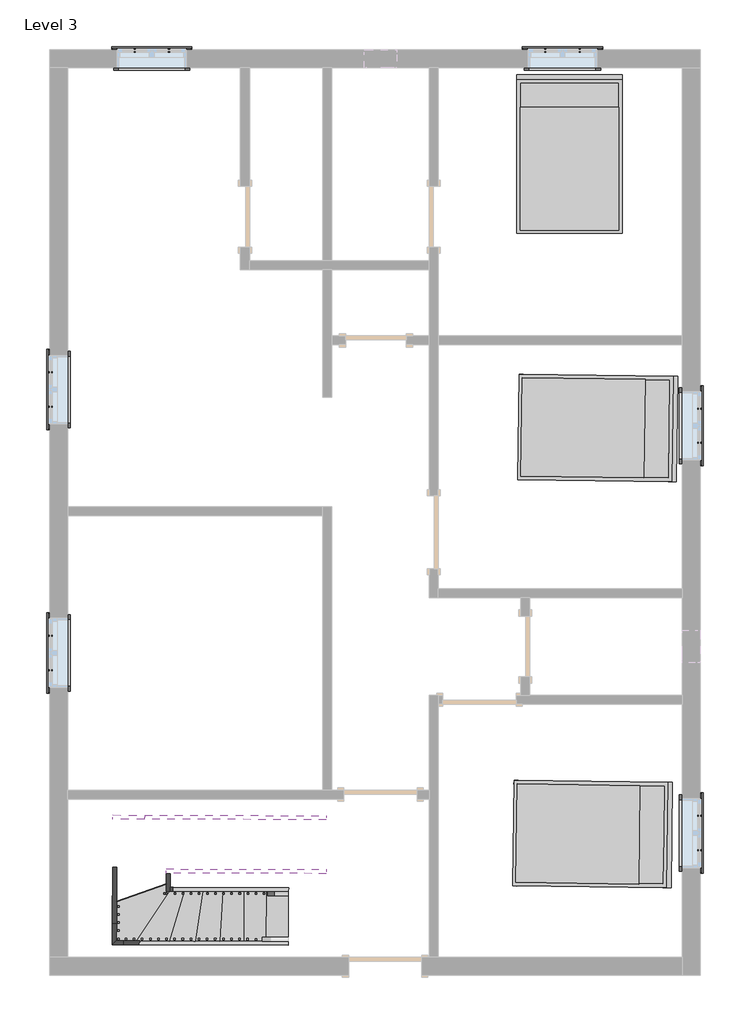
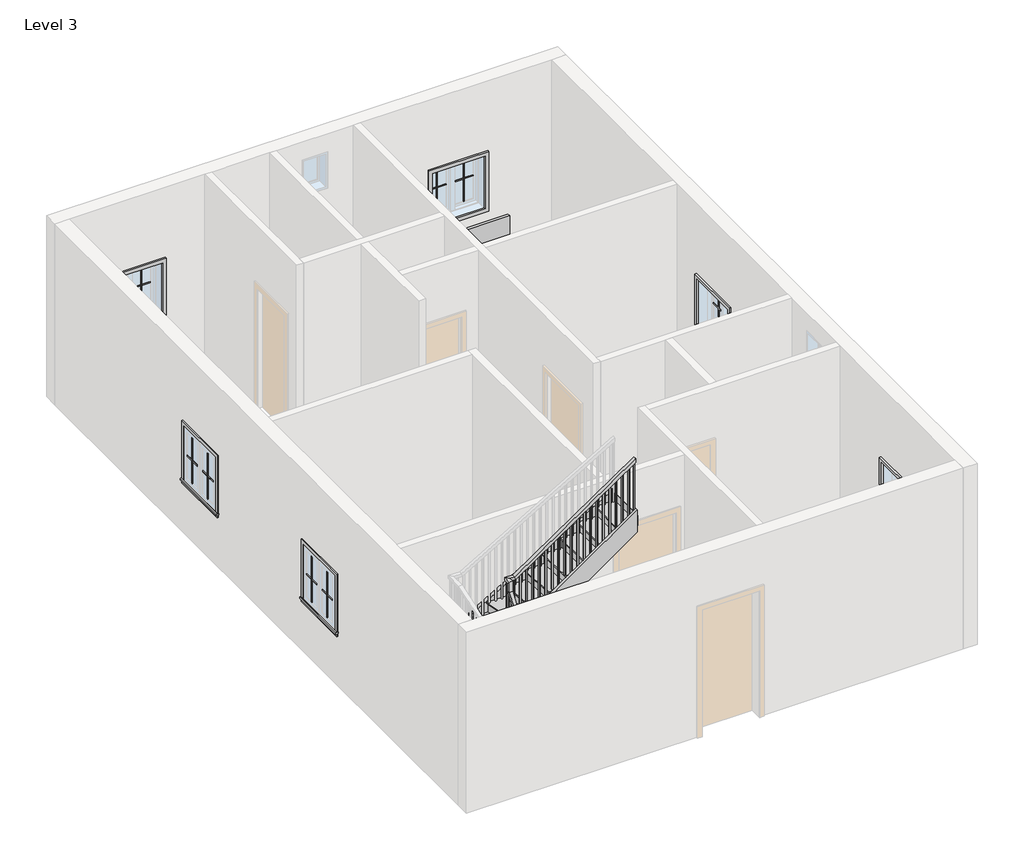
# One storey, part 3 of 3: 24 proxies, 9 members, 3 furniture elements, 1 railing, 1 stair flight.
"""IFC4 building model written with IfcOpenShell, lengths in millimetres."""

from ifc_helpers import new_model, si_unit, frame, origin, place, context, project, spatial, polyline, outline, extrude, faceted_brep, transform, mapped, element, save
from components import muntin_pattern_2x2_muntin_pattern_2x2_b3fe6957, muntin_pattern_2x2_muntin_pattern_2x2_3e0ecaf2, trim_window_exterior_flat_with_sill_41619996, trim_window_interior_flat_picture_frame_51c85655, bed_17739_bed_17739_15c61121, stair_flight_9e3aa5cb

model = new_model("IFC4")

# Units and contexts
model_context = context("Model", 3, world=origin())
ifc_project = project(units=[si_unit("LENGTHUNIT", "METRE", prefix="MILLI")], contexts=[model_context])

# Site, building, storey
site = spatial("IfcSite", under=ifc_project)
building = spatial("IfcBuilding", under=site)
storey = spatial("IfcBuildingStorey", under=building, Name="Level 3", Elevation=3200.4)

# Proxies
placement = place(None, origin())
muntin_pattern_2x2_muntin_pattern_2x2_shape = muntin_pattern_2x2_muntin_pattern_2x2_b3fe6957(model_context)
element("IfcBuildingElementProxy", 1, Name="Muntin Pattern_2x2 : Muntin Pattern_2x2", ObjectType="Muntin Pattern_2x2 : Muntin Pattern_2x2", at=placement, inside=storey, context=model_context, shape_type="MappedRepresentation", body=[
    mapped(muntin_pattern_2x2_muntin_pattern_2x2_shape, transform((873.7257686, 6321.6571212, 4184.65), x_axis=(1.0, 0.0, 0.0), y_axis=(0.0, 1.0, 0.0), z_axis=(0.0, 0.0, 1.0))),
])
element("IfcBuildingElementProxy", 2, Name="Muntin Pattern_2x2 : Muntin Pattern_2x2", ObjectType="Muntin Pattern_2x2 : Muntin Pattern_2x2", at=placement, inside=storey, context=model_context, shape_type="MappedRepresentation", body=[
    mapped(muntin_pattern_2x2_muntin_pattern_2x2_shape, transform((2802.5382686, 1840.1446212, 4184.65), x_axis=(0.0, -1.0, 0.0), y_axis=(1.0, 0.0, 0.0), z_axis=(0.0, 0.0, 1.0))),
])
element("IfcBuildingElementProxy", 3, Name="Muntin Pattern_2x2 : Muntin Pattern_2x2", ObjectType="Muntin Pattern_2x2 : Muntin Pattern_2x2", at=placement, inside=storey, context=model_context, shape_type="MappedRepresentation", body=[
    mapped(muntin_pattern_2x2_muntin_pattern_2x2_shape, transform((2802.5382686, -3255.7303788, 4184.65), x_axis=(0.0, -1.0, 0.0), y_axis=(1.0, 0.0, 0.0), z_axis=(0.0, 0.0, 1.0))),
])
element("IfcBuildingElementProxy", 4, Name="Muntin Pattern_2x2 : Muntin Pattern_2x2", ObjectType="Muntin Pattern_2x2 : Muntin Pattern_2x2", at=placement, inside=storey, context=model_context, shape_type="MappedRepresentation", body=[
    mapped(muntin_pattern_2x2_muntin_pattern_2x2_shape, transform((-4263.4242314, 6321.6571212, 4184.65), x_axis=(1.0, 0.0, 0.0), y_axis=(0.0, 1.0, 0.0), z_axis=(0.0, 0.0, 1.0))),
])
element("IfcBuildingElementProxy", 5, Name="Muntin Pattern_2x2 : Muntin Pattern_2x2", ObjectType="Muntin Pattern_2x2 : Muntin Pattern_2x2", at=placement, inside=storey, context=model_context, shape_type="MappedRepresentation", body=[
    mapped(muntin_pattern_2x2_muntin_pattern_2x2_shape, transform((-5319.1117314, 1863.8332318, 4184.65), x_axis=(0.0, 1.0, 0.0), y_axis=(-1.0, 0.0, 0.0), z_axis=(0.0, 0.0, 1.0))),
])
element("IfcBuildingElementProxy", 6, Name="Muntin Pattern_2x2 : Muntin Pattern_2x2", ObjectType="Muntin Pattern_2x2 : Muntin Pattern_2x2", at=placement, inside=storey, context=model_context, shape_type="MappedRepresentation", body=[
    mapped(muntin_pattern_2x2_muntin_pattern_2x2_shape, transform((-5319.1117314, -1431.8167682, 4184.65), x_axis=(0.0, 1.0, 0.0), y_axis=(-1.0, 0.0, 0.0), z_axis=(0.0, 0.0, 1.0))),
])
muntin_pattern_2x2_muntin_pattern_2x2_2_shape = muntin_pattern_2x2_muntin_pattern_2x2_3e0ecaf2(model_context)
element("IfcBuildingElementProxy", 7, Name="Muntin Pattern_2x2 : Muntin Pattern_2x2", ObjectType="Muntin Pattern_2x2 : Muntin Pattern_2x2", at=placement, inside=storey, context=model_context, shape_type="MappedRepresentation", body=[
    mapped(muntin_pattern_2x2_muntin_pattern_2x2_2_shape, transform((1302.3507686, 6321.6571212, 4184.65), x_axis=(-1.0, 0.0, 0.0), y_axis=(0.0, -1.0, 0.0), z_axis=(0.0, 0.0, 1.0))),
])
element("IfcBuildingElementProxy", 8, Name="Muntin Pattern_2x2 : Muntin Pattern_2x2", ObjectType="Muntin Pattern_2x2 : Muntin Pattern_2x2", at=placement, inside=storey, context=model_context, shape_type="MappedRepresentation", body=[
    mapped(muntin_pattern_2x2_muntin_pattern_2x2_2_shape, transform((2802.5382686, 1411.5196212, 4184.65), x_axis=(0.0, 1.0, 0.0), y_axis=(-1.0, 0.0, 0.0), z_axis=(0.0, 0.0, 1.0))),
])
element("IfcBuildingElementProxy", 9, Name="Muntin Pattern_2x2 : Muntin Pattern_2x2", ObjectType="Muntin Pattern_2x2 : Muntin Pattern_2x2", at=placement, inside=storey, context=model_context, shape_type="MappedRepresentation", body=[
    mapped(muntin_pattern_2x2_muntin_pattern_2x2_2_shape, transform((2802.5382686, -3684.3553788, 4184.65), x_axis=(0.0, 1.0, 0.0), y_axis=(-1.0, 0.0, 0.0), z_axis=(0.0, 0.0, 1.0))),
])
element("IfcBuildingElementProxy", 10, Name="Muntin Pattern_2x2 : Muntin Pattern_2x2", ObjectType="Muntin Pattern_2x2 : Muntin Pattern_2x2", at=placement, inside=storey, context=model_context, shape_type="MappedRepresentation", body=[
    mapped(muntin_pattern_2x2_muntin_pattern_2x2_2_shape, transform((-3834.7992314, 6321.6571212, 4184.65), x_axis=(-1.0, 0.0, 0.0), y_axis=(0.0, -1.0, 0.0), z_axis=(0.0, 0.0, 1.0))),
])
element("IfcBuildingElementProxy", 11, Name="Muntin Pattern_2x2 : Muntin Pattern_2x2", ObjectType="Muntin Pattern_2x2 : Muntin Pattern_2x2", at=placement, inside=storey, context=model_context, shape_type="MappedRepresentation", body=[
    mapped(muntin_pattern_2x2_muntin_pattern_2x2_2_shape, transform((-5319.1117314, 2292.4582318, 4184.65), x_axis=(0.0, -1.0, 0.0), y_axis=(1.0, 0.0, 0.0), z_axis=(0.0, 0.0, 1.0))),
])
element("IfcBuildingElementProxy", 12, Name="Muntin Pattern_2x2 : Muntin Pattern_2x2", ObjectType="Muntin Pattern_2x2 : Muntin Pattern_2x2", at=placement, inside=storey, context=model_context, shape_type="MappedRepresentation", body=[
    mapped(muntin_pattern_2x2_muntin_pattern_2x2_2_shape, transform((-5319.1117314, -1003.1917682, 4184.65), x_axis=(0.0, -1.0, 0.0), y_axis=(1.0, 0.0, 0.0), z_axis=(0.0, 0.0, 1.0))),
])
trim_window_exterior_flat_with_sill_shape = trim_window_exterior_flat_with_sill_41619996(model_context)
element("IfcBuildingElementProxy", 13, Name="Trim-Window-Exterior-Flat : with Sill", ObjectType="Trim-Window-Exterior-Flat : with Sill", at=placement, inside=storey, context=model_context, shape_type="MappedRepresentation", body=[
    mapped(trim_window_exterior_flat_with_sill_shape, transform((1088.0382686, 6331.1821212, 5029.2), x_axis=(-1.0, 0.0, 0.0), y_axis=(0.0, 0.0, 1.0), z_axis=(0.0, 1.0, 0.0))),
])
element("IfcBuildingElementProxy", 14, Name="Trim-Window-Exterior-Flat : with Sill", ObjectType="Trim-Window-Exterior-Flat : with Sill", at=placement, inside=storey, context=model_context, shape_type="MappedRepresentation", body=[
    mapped(trim_window_exterior_flat_with_sill_shape, transform((2812.0632686, 1625.8321212, 5029.2), x_axis=(0.0, 1.0, 0.0), y_axis=(0.0, 0.0, 1.0), z_axis=(1.0, 0.0, 0.0))),
])
element("IfcBuildingElementProxy", 15, Name="Trim-Window-Exterior-Flat : with Sill", ObjectType="Trim-Window-Exterior-Flat : with Sill", at=placement, inside=storey, context=model_context, shape_type="MappedRepresentation", body=[
    mapped(trim_window_exterior_flat_with_sill_shape, transform((2812.0632686, -3470.0428788, 5029.2), x_axis=(0.0, 1.0, 0.0), y_axis=(0.0, 0.0, 1.0), z_axis=(1.0, 0.0, 0.0))),
])
element("IfcBuildingElementProxy", 16, Name="Trim-Window-Exterior-Flat : with Sill", ObjectType="Trim-Window-Exterior-Flat : with Sill", at=placement, inside=storey, context=model_context, shape_type="MappedRepresentation", body=[
    mapped(trim_window_exterior_flat_with_sill_shape, transform((-4049.1117314, 6331.1821212, 5029.2), x_axis=(-1.0, 0.0, 0.0), y_axis=(0.0, 0.0, 1.0), z_axis=(0.0, 1.0, 0.0))),
])
element("IfcBuildingElementProxy", 17, Name="Trim-Window-Exterior-Flat : with Sill", ObjectType="Trim-Window-Exterior-Flat : with Sill", at=placement, inside=storey, context=model_context, shape_type="MappedRepresentation", body=[
    mapped(trim_window_exterior_flat_with_sill_shape, transform((-5328.6367314, 2078.1457318, 5029.2), x_axis=(0.0, -1.0, 0.0), y_axis=(0.0, 0.0, 1.0), z_axis=(-1.0, 0.0, 0.0))),
])
element("IfcBuildingElementProxy", 18, Name="Trim-Window-Exterior-Flat : with Sill", ObjectType="Trim-Window-Exterior-Flat : with Sill", at=placement, inside=storey, context=model_context, shape_type="MappedRepresentation", body=[
    mapped(trim_window_exterior_flat_with_sill_shape, transform((-5328.6367314, -1217.5042682, 5029.2), x_axis=(0.0, -1.0, 0.0), y_axis=(0.0, 0.0, 1.0), z_axis=(-1.0, 0.0, 0.0))),
])
trim_window_interior_flat_picture_frame_shape = trim_window_interior_flat_picture_frame_51c85655(model_context)
element("IfcBuildingElementProxy", 19, Name="Trim-Window-Interior-Flat : Picture Frame", ObjectType="Trim-Window-Interior-Flat : Picture Frame", at=placement, inside=storey, context=model_context, shape_type="MappedRepresentation", body=[
    mapped(trim_window_interior_flat_picture_frame_shape, transform((1088.0382686, 6102.5821212, 5029.2), x_axis=(1.0, 0.0, 0.0), y_axis=(0.0, 0.0, 1.0), z_axis=(0.0, -1.0, 0.0))),
])
element("IfcBuildingElementProxy", 20, Name="Trim-Window-Interior-Flat : Picture Frame", ObjectType="Trim-Window-Interior-Flat : Picture Frame", at=placement, inside=storey, context=model_context, shape_type="MappedRepresentation", body=[
    mapped(trim_window_interior_flat_picture_frame_shape, transform((2583.4632686, 1625.8321212, 5029.2), x_axis=(0.0, -1.0, 0.0), y_axis=(0.0, 0.0, 1.0), z_axis=(-1.0, 0.0, 0.0))),
])
element("IfcBuildingElementProxy", 21, Name="Trim-Window-Interior-Flat : Picture Frame", ObjectType="Trim-Window-Interior-Flat : Picture Frame", at=placement, inside=storey, context=model_context, shape_type="MappedRepresentation", body=[
    mapped(trim_window_interior_flat_picture_frame_shape, transform((2583.4632686, -3470.0428788, 5029.2), x_axis=(0.0, -1.0, 0.0), y_axis=(0.0, 0.0, 1.0), z_axis=(-1.0, 0.0, 0.0))),
])
element("IfcBuildingElementProxy", 22, Name="Trim-Window-Interior-Flat : Picture Frame", ObjectType="Trim-Window-Interior-Flat : Picture Frame", at=placement, inside=storey, context=model_context, shape_type="MappedRepresentation", body=[
    mapped(trim_window_interior_flat_picture_frame_shape, transform((-4049.1117314, 6102.5821212, 5029.2), x_axis=(1.0, 0.0, 0.0), y_axis=(0.0, 0.0, 1.0), z_axis=(0.0, -1.0, 0.0))),
])
element("IfcBuildingElementProxy", 23, Name="Trim-Window-Interior-Flat : Picture Frame", ObjectType="Trim-Window-Interior-Flat : Picture Frame", at=placement, inside=storey, context=model_context, shape_type="MappedRepresentation", body=[
    mapped(trim_window_interior_flat_picture_frame_shape, transform((-5100.0367314, 2078.1457318, 5029.2), x_axis=(0.0, 1.0, 0.0), y_axis=(0.0, 0.0, 1.0), z_axis=(1.0, 0.0, 0.0))),
])
element("IfcBuildingElementProxy", 24, Name="Trim-Window-Interior-Flat : Picture Frame", ObjectType="Trim-Window-Interior-Flat : Picture Frame", at=placement, inside=storey, context=model_context, shape_type="MappedRepresentation", body=[
    mapped(trim_window_interior_flat_picture_frame_shape, transform((-5100.0367314, -1217.5042682, 5029.2), x_axis=(0.0, 1.0, 0.0), y_axis=(0.0, 0.0, 1.0), z_axis=(1.0, 0.0, 0.0))),
])

# Furniture
bed_17739_bed_17739_shape = bed_17739_bed_17739_15c61121(model_context)
element("IfcFurniture", 25, ObjectType="Bed_17739 : Bed_17739", at=placement, inside=storey, context=model_context, shape_type="MappedRepresentation", body=[
    mapped(bed_17739_bed_17739_shape, transform((1173.7632686, 4997.6821212, 3200.4), x_axis=(1.0, 0.0, 0.0), y_axis=(0.0, 1.0, 0.0), z_axis=(0.0, 0.0, 1.0))),
])
element("IfcFurniture", 26, ObjectType="Bed_17739 : Bed_17739", at=placement, inside=storey, context=model_context, shape_type="MappedRepresentation", body=[
    mapped(bed_17739_bed_17739_shape, transform((1503.3372561, 1596.4447738, 3200.4), x_axis=(-0.012740965827000846, -0.9999188306006619, 0.0), y_axis=(0.9999188306006619, -0.012740965827000846, 0.0), z_axis=(0.0, 0.0, 1.0))),
])
element("IfcFurniture", 27, ObjectType="Bed_17739 : Bed_17739", at=placement, inside=storey, context=model_context, shape_type="MappedRepresentation", body=[
    mapped(bed_17739_bed_17739_shape, transform((1438.6034215, -3483.9063624, 3200.4), x_axis=(-0.012740965827007402, -0.9999188306006618, 0.0), y_axis=(0.9999188306006618, -0.012740965827007402, 0.0), z_axis=(0.0, 0.0, 1.0))),
])

# Members
element("IfcMember", 28, ObjectType="Stringer - 2\" Width", at=placement, inside=storey, context=model_context, shape_type="SweptSolid", body=[
    extrude(outline(polyline([(-105.6436802, -202.41926), (0.0, 0.0), (2328.0658822, 0.0), (2168.9891534, -304.7999999), (90.5236019, -304.7999999), (-105.6436802, -202.41926)])), frame((-2342.1993001, -4876.8012848, 3428.7290257), z_axis=(0.0033835818014385714, 0.9999942756707126, 0.0), x_axis=(-0.8865193579369283, 0.0029996279369964417, 0.46268178074713084)), (0.0, 0.0, 1.0), 50.8),
])
element("IfcMember", 29, ObjectType="Stringer - 2\" Width", at=placement, inside=storey, context=model_context, shape_type="SweptSolid", body=[
    extrude(outline(polyline([(-4405.9028852, -4819.0182441), (-4406.0747712, -4869.8179533), (-4542.6986856, -4869.3556725), (-4491.7270905, -4818.7278493), (-4405.9028852, -4819.0182441)])), frame((0.0, 0.0, 4162.0681426), z_axis=(0.0, 0.0, 1.0), x_axis=(1.0, 0.0, 0.0)), (0.0, 0.0, 1.0), 343.8145513),
])
element("IfcMember", 30, ObjectType="Stringer - 2\" Width", at=placement, inside=storey, context=model_context, shape_type="SweptSolid", body=[
    extrude(outline(polyline([(-4491.7270905, -4818.7278493), (-4542.6986856, -4869.3556725), (-4541.8102896, -4606.7963526), (-4491.0105804, -4606.9682386), (-4491.7270905, -4818.7278493)])), frame((0.0, 0.0, 4162.0681426), z_axis=(0.0, 0.0, 1.0), x_axis=(1.0, 0.0, 0.0)), (0.0, 0.0, 1.0), 343.8145513),
])
element("IfcMember", 31, ObjectType="Stringer - 2\" Width", at=placement, inside=storey, context=model_context, shape_type="SweptSolid", body=[
    extrude(outline(polyline([(109.7110974, -325.8403301), (0.0, 0.0), (1383.9510961, 0.0), (1489.930143, -314.7561954), (1457.0104275, -325.8403301), (109.7110974, -325.8403301)])), frame((-4491.0105804, -4606.9682386, 4162.0681426), z_axis=(-0.9999942756707125, 0.003383581801438886, 0.0), x_axis=(0.0032066921171017464, 0.9477157489074122, 0.3190996339680272)), (0.0, 0.0, 1.0), 50.8),
])
element("IfcMember", 32, ObjectType="Stringer - 2\" Width", at=placement, inside=storey, context=model_context, shape_type="SweptSolid", body=[
    extrude(outline(polyline([(-4537.3723845, -3295.2041032), (-4537.2004986, -3244.404394), (-4139.0142012, -3245.7516976), (-4139.1860871, -3296.5514068), (-4537.3723845, -3295.2041032)])), frame((0.0, 0.0, 4614.1918365), z_axis=(0.0, 0.0, 1.0), x_axis=(1.0, 0.0, 0.0)), (0.0, 0.0, 1.0), 321.6135804),
])
element("IfcMember", 33, ObjectType="Stringer - 2\" Width", at=placement, inside=storey, context=model_context, shape_type="SweptSolid", body=[
    extrude(outline(polyline([(-111.9549294, -160.635527), (0.0, 0.0), (1800.2454177, 0.0), (1587.8150598, -304.8000001), (94.8955973, -304.8), (-111.9549294, -160.635527)])), frame((-2339.9228929, -4204.0248458, 3396.2000989), z_axis=(0.003383581801438833, 0.9999942756707125, 0.0), x_axis=(-0.8204010535979692, 0.0027759099650580456, 0.5717817814334486)), (0.0, 0.0, 1.0), 50.8),
])
element("IfcMember", 34, ObjectType="Stringer - 2\" Width", at=placement, inside=storey, context=model_context, shape_type="SweptSolid", body=[
    extrude(outline(polyline([(438.5777673, -304.8), (2.5808594, -1.7936294), (3.8273846, 0.0), (400.5684618, 0.0), (819.8223258, -291.370396), (810.4891046, -304.8000001), (438.5777673, -304.8)])), frame((-3816.8461303, -4199.0275266, 4086.2862902), z_axis=(-0.9999942756707125, 0.003383581801437359, 0.0), x_axis=(0.0019309727886812926, 0.5706856959500506, 0.8211663094538743)), (0.0, 0.0, 1.0), 50.8),
])
element("IfcMember", 35, ObjectType="Stringer - 2\" Width", at=placement, inside=storey, context=model_context, shape_type="SweptSolid", body=[
    extrude(outline(polyline([(213.8292849, -304.8), (0.0, 0.0), (2440.5867528, 0.0), (2654.4160377, -304.8), (213.8292849, -304.8)])), frame((-3866.8723527, -3970.2569493, 4553.4535021), z_axis=(0.003383581801438697, 0.9999942756707126, 0.0), x_axis=(0.8186346554264393, -0.0027699331781375542, 0.5743079560697587)), (0.0, 0.0, 1.0), 50.8),
])
element("IfcMember", 36, ObjectType="Stringer - 2\" Width", at=placement, inside=storey, context=model_context, shape_type="SweptSolid", body=[
    extrude(outline(polyline([(162.5062199, -277.5374274), (0.0, 0.0), (2633.4595913, 1e-07), (2795.9658112, -277.5374274), (162.5062199, -277.5374274)])), frame((-4139.1860871, -3296.5514068, 4614.1918365), z_axis=(0.0033835818014385927, 0.9999942756707125, 0.0), x_axis=(0.8629481327443969, -0.002919872311849946, 0.5052840731100094)), (0.0, 0.0, 1.0), 50.8),
])

# Railing
element("IfcRailing", 37, ObjectType="Handrail - Rectangular", at=placement, inside=storey, context=model_context, shape_type="SolidModel", body=[
    faceted_brep([(-2340.0947789, -4254.824555, 4284.1333333), (-2340.0947789, -4254.824555, 4222.7023206), (-2339.9228929, -4204.0248458, 4222.7023206), (-2339.9228929, -4204.0248458, 4284.1333333), (-3791.6181617, -4249.9131788, 5271.1092848), (-3842.4178709, -4249.7412929, 5244.2199762), (-3842.2459849, -4198.9415837, 5244.2199762), (-3791.4462757, -4199.1134696, 5271.1092848), (-1868.5796854, -3875.4177931, 7162.8), (-1868.7515713, -3926.2175023, 7162.8), (-1868.7515713, -3926.2175023, 7101.138507), (-1868.5796854, -3875.4177931, 7101.138507), (-3774.5418549, -3868.9687773, 5789.845528), (-3790.329017, -3868.9153598, 5840.645528), (-3774.7137409, -3919.7684865, 5789.845528), (-3790.500903, -3919.715069, 5840.645528), (-3791.6181617, -4249.9131788, 5487.4182666), (-3842.4178709, -4249.7412929, 5436.6182666), (-3842.2459849, -4198.9415837, 5436.6182666), (-3791.4462757, -4199.1134696, 5487.4182666), (-3918.6174347, -4249.4834639, 5487.4182666), (-3918.6174347, -4249.4834639, 5436.6182666), (-3867.6458395, -4198.8556407, 5436.6182666), (-3867.6458395, -4198.8556407, 5487.4182666), (-3918.1877198, -4122.4841909, 5487.4182666), (-3918.0978567, -4095.9257757, 5436.6182666), (-3867.2981475, -4096.0976616, 5436.6182666), (-3867.3880106, -4122.6560769, 5487.4182666), (-3917.7580049, -3995.4849179, 5670.159003), (-3917.586119, -3944.6852087, 5654.2400838), (-3866.7864097, -3944.8570947, 5654.2400838), (-3866.9582957, -3995.6568039, 5670.159003), (-3917.7580049, -3995.4849179, 5840.645528), (-3917.586119, -3944.6852087, 5789.845528), (-3866.7864097, -3944.8570947, 5789.845528), (-3866.9582957, -3995.6568039, 5840.645528), (-3917.32829, -3868.4856449, 5840.645528), (-3917.32829, -3868.4856449, 5789.845528), (-3866.7004668, -3919.4572401, 5789.845528), (-3866.7004668, -3919.4572401, 5840.645528)], [[[0, 1, 2, 3]], [[1, 0, 4, 5]], [[2, 1, 5, 6]], [[3, 2, 6, 7]], [[0, 3, 7, 4]], [[8, 9, 10, 11]], [[12, 13, 8, 11]], [[14, 12, 11, 10]], [[15, 14, 10, 9]], [[13, 15, 9, 8]], [[5, 4, 16, 17]], [[6, 5, 17, 18]], [[7, 6, 18, 19]], [[4, 7, 19, 16]], [[17, 16, 20, 21]], [[18, 17, 21, 22]], [[19, 18, 22, 23]], [[16, 19, 23, 20]], [[21, 20, 24, 25]], [[22, 21, 25, 26]], [[23, 22, 26, 27]], [[20, 23, 27, 24]], [[25, 24, 28, 29]], [[26, 25, 29, 30]], [[27, 26, 30, 31]], [[24, 27, 31, 28]], [[29, 28, 32, 33]], [[30, 29, 33, 34]], [[31, 30, 34, 35]], [[28, 31, 35, 32]], [[33, 32, 36, 37]], [[34, 33, 37, 38]], [[35, 34, 38, 39]], [[32, 35, 39, 36]], [[37, 36, 13, 12]], [[38, 37, 12, 14]], [[39, 38, 14, 15]], [[36, 39, 15, 13]]]),
    extrude(outline(polyline([(222.0468824, -19.0499999), (235.1531175, 0.0), (1186.7159363, 0.0), (1186.7159363, -19.0499999), (222.0468824, -19.0499999)])), frame((-1971.1826027, -3909.9958257, 7265.782603), z_axis=(0.0033835818014386967, 0.9999942756707125, 0.0), x_axis=(0.0, 0.0, -1.0)), (0.0, 0.0, 1.0), 19.05),
    extrude(outline(polyline([(222.0468825, -19.0499999), (235.1531175, 0.0), (1116.8160159, 0.0), (1116.8160159, -19.0499999), (222.0468825, -19.0499999)])), frame((-2072.7820211, -3909.6520537, 7195.8826826), z_axis=(0.0033835818014386967, 0.9999942756707125, 0.0), x_axis=(0.0, 0.0, -1.0)), (0.0, 0.0, 1.0), 19.05),
    extrude(outline(polyline([(222.0468825, -19.0499999), (235.1531176, 0.0), (1216.2494289, 0.0), (1216.2494289, -19.0499999), (222.0468825, -19.0499999)])), frame((-2174.3814395, -3909.3082818, 7125.9827622), z_axis=(0.0033835818014386967, 0.9999942756707125, 0.0), x_axis=(0.0, 0.0, -1.0)), (0.0, 0.0, 1.0), 19.05),
    extrude(outline(polyline([(222.0468825, -19.05), (235.1531175, 0.0), (1146.3495084, 0.0), (1146.3495084, -19.05), (222.0468825, -19.05)])), frame((-2275.980858, -3908.9645099, 7056.0828417), z_axis=(0.0033835818014386967, 0.9999942756707125, 0.0), x_axis=(0.0, 0.0, -1.0)), (0.0, 0.0, 1.0), 19.05),
    extrude(outline(polyline([(222.0468825, -19.05), (235.1531176, 0.0), (1076.449588, 0.0), (1076.449588, -19.05), (222.0468825, -19.05)])), frame((-2377.5802764, -3908.620738, 6986.1829213), z_axis=(0.0033835818014386967, 0.9999942756707125, 0.0), x_axis=(0.0, 0.0, -1.0)), (0.0, 0.0, 1.0), 19.05),
    extrude(outline(polyline([(222.0468824, -19.05), (235.1531175, 0.0), (1175.8830008, 0.0), (1175.8830008, -19.05), (222.0468824, -19.05)])), frame((-2479.1796948, -3908.2769661, 6916.2830008), z_axis=(0.0033835818014386967, 0.9999942756707125, 0.0), x_axis=(0.0, 0.0, -1.0)), (0.0, 0.0, 1.0), 19.05),
    extrude(outline(polyline([(222.0468825, -19.05), (235.1531176, 0.0), (1105.9830804, 0.0), (1105.9830804, -19.05), (222.0468825, -19.05)])), frame((-2580.7791132, -3907.9331942, 6846.3830804), z_axis=(0.0033835818014386967, 0.9999942756707125, 0.0), x_axis=(0.0, 0.0, -1.0)), (0.0, 0.0, 1.0), 19.05),
    extrude(outline(polyline([(222.0468824, -19.05), (235.1531175, 0.0), (1036.0831599, 0.0), (1036.0831599, -19.05), (222.0468824, -19.05)])), frame((-2682.3785316, -3907.5894223, 6776.4831599), z_axis=(0.0033835818014386967, 0.9999942756707125, 0.0), x_axis=(0.0, 0.0, -1.0)), (0.0, 0.0, 1.0), 19.05),
    extrude(outline(polyline([(222.0468825, -19.05), (235.1531176, 0.0), (1135.5165728, 0.0), (1135.5165728, -19.05), (222.0468825, -19.05)])), frame((-2783.97795, -3907.2456504, 6706.5832395), z_axis=(0.0033835818014386967, 0.9999942756707125, 0.0), x_axis=(0.0, 0.0, -1.0)), (0.0, 0.0, 1.0), 19.05),
    extrude(outline(polyline([(222.0468824, -19.0499999), (235.1531175, 0.0), (1065.6166523, 0.0), (1065.6166523, -19.0499999), (222.0468824, -19.0499999)])), frame((-2885.5773684, -3906.9018785, 6636.683319), z_axis=(0.0033835818014386967, 0.9999942756707125, 0.0), x_axis=(0.0, 0.0, -1.0)), (0.0, 0.0, 1.0), 19.05),
    extrude(outline(polyline([(222.0468825, -19.0499999), (235.1531176, 0.0), (995.7167319, 0.0), (995.7167319, -19.0499999), (222.0468825, -19.0499999)])), frame((-2987.1767868, -3906.5581065, 6566.7833986), z_axis=(0.0033835818014386967, 0.9999942756707125, 0.0), x_axis=(0.0, 0.0, -1.0)), (0.0, 0.0, 1.0), 19.05),
    extrude(outline(polyline([(222.0468824, -19.0499999), (235.1531175, 0.0), (1095.1501448, 0.0), (1095.1501448, -19.0499999), (222.0468824, -19.0499999)])), frame((-3088.7762052, -3906.2143346, 6496.8834781), z_axis=(0.0033835818014386967, 0.9999942756707125, 0.0), x_axis=(0.0, 0.0, -1.0)), (0.0, 0.0, 1.0), 19.05),
    extrude(outline(polyline([(222.0468825, -19.0499999), (235.1531176, 0.0), (1025.2502244, 0.0), (1025.2502244, -19.0499999), (222.0468825, -19.0499999)])), frame((-3190.3756236, -3905.8705627, 6426.9835577), z_axis=(0.0033835818014386967, 0.9999942756707125, 0.0), x_axis=(0.0, 0.0, -1.0)), (0.0, 0.0, 1.0), 19.05),
    extrude(outline(polyline([(222.0468824, -19.0499999), (235.1531175, 0.0), (1124.6836372, 0.0), (1124.6836372, -19.0499999), (222.0468824, -19.0499999)])), frame((-3291.975042, -3905.5267908, 6357.0836372), z_axis=(0.0033835818014386967, 0.9999942756707125, 0.0), x_axis=(0.0, 0.0, -1.0)), (0.0, 0.0, 1.0), 19.05),
    extrude(outline(polyline([(222.0468825, -19.0499999), (235.1531176, 0.0), (1054.7837168, 0.0), (1054.7837168, -19.0499999), (222.0468825, -19.0499999)])), frame((-3393.5744604, -3905.1830189, 6287.1837168), z_axis=(0.0033835818014386967, 0.9999942756707125, 0.0), x_axis=(0.0, 0.0, -1.0)), (0.0, 0.0, 1.0), 19.05),
    extrude(outline(polyline([(222.0468824, -19.05), (235.1531175, 0.0), (984.8837963, 0.0), (984.8837963, -19.05), (222.0468824, -19.05)])), frame((-3495.1738789, -3904.839247, 6217.2837963), z_axis=(0.0033835818014386967, 0.9999942756707125, 0.0), x_axis=(0.0, 0.0, -1.0)), (0.0, 0.0, 1.0), 19.05),
    extrude(outline(polyline([(222.0468825, -19.05), (235.1531176, 0.0), (1084.3172092, 0.0), (1084.3172092, -19.05), (222.0468825, -19.05)])), frame((-3596.7732973, -3904.4954751, 6147.3838759), z_axis=(0.0033835818014386967, 0.9999942756707125, 0.0), x_axis=(0.0, 0.0, -1.0)), (0.0, 0.0, 1.0), 19.05),
    extrude(outline(polyline([(222.0468824, -19.05), (235.1531175, 0.0), (1014.4172887, 0.0), (1014.4172887, -19.05), (222.0468824, -19.05)])), frame((-3698.3727157, -3904.1517032, 6077.4839554), z_axis=(0.0033835818014386967, 0.9999942756707125, 0.0), x_axis=(0.0, 0.0, -1.0)), (0.0, 0.0, 1.0), 19.05),
    extrude(outline(polyline([(222.0468825, -19.05), (235.1531175, 0.0), (1113.8507017, 0.0), (1113.8507017, -19.05), (222.0468825, -19.05)])), frame((-3799.9721341, -3903.8079313, 6007.584035), z_axis=(0.0033835818014386967, 0.9999942756707125, 0.0), x_axis=(0.0, 0.0, -1.0)), (0.0, 0.0, 1.0), 19.05),
    extrude(outline(polyline([(-3882.6076045, -3928.9284712), (-3901.6574955, -3928.8640139), (-3901.5930382, -3909.814123), (-3882.5431473, -3909.8785802), (-3882.6076045, -3928.9284712)])), frame((0.0, 0.0, 4724.4), z_axis=(0.0, 0.0, 1.0), x_axis=(1.0, 0.0, 0.0)), (0.0, 0.0, 1.0), 1065.445528),
    extrude(outline(polyline([(214.8944448, -19.05), (242.3055552, 0.0), (1218.1289753, 0.0), (1218.1289753, -19.05), (214.8944448, -19.05)])), frame((-3882.9513764, -4030.5278896, 5773.195642), z_axis=(-0.9999942756707125, 0.0033835818014373593, 0.0), x_axis=(0.0, 0.0, -1.0)), (0.0, 0.0, 1.0), 19.05),
    extrude(outline(polyline([(214.8944448, -19.05), (242.3055552, 0.0), (1071.9363862, 0.0), (1071.9363862, -19.05), (214.8944448, -19.05)])), frame((-3883.2951483, -4132.127308, 5627.0030529), z_axis=(-0.9999942756707125, 0.0033835818014373593, 0.0), x_axis=(0.0, 0.0, -1.0)), (0.0, 0.0, 1.0), 19.05),
    extrude(outline(polyline([(-3854.4429379, -4214.7754049), (-3854.5073951, -4233.8252959), (-3873.5572861, -4233.7608386), (-3873.4928289, -4214.7109477), (-3854.4429379, -4214.7754049)])), frame((0.0, 0.0, 4385.7333333), z_axis=(0.0, 0.0, 1.0), x_axis=(1.0, 0.0, 0.0)), (0.0, 0.0, 1.0), 1050.8849333),
    extrude(outline(polyline([(235.0765695, -19.05), (222.1234305, 0.0), (1202.0700381, 0.0), (1202.0700381, -19.05), (235.0765695, -19.05)])), frame((-3771.9578677, -4234.1046105, 5418.4700381), z_axis=(0.003383581801438833, 0.9999942756707125, 0.0), x_axis=(0.0, 0.0, -1.0)), (0.0, 0.0, 1.0), 19.05),
    extrude(outline(polyline([(235.0765695, -19.05), (222.1234305, 0.0), (1132.9866297, 0.0), (1132.9866297, -19.05), (235.0765695, -19.05)])), frame((-3670.3584493, -4234.4483825, 5349.3866297), z_axis=(0.003383581801438833, 0.9999942756707125, 0.0), x_axis=(0.0, 0.0, -1.0)), (0.0, 0.0, 1.0), 19.05),
    extrude(outline(polyline([(235.0765695, -19.05), (222.1234305, 0.0), (1233.2365546, 0.0), (1233.2365546, -19.05), (235.0765695, -19.05)])), frame((-3568.7590309, -4234.7921544, 5280.3032213), z_axis=(0.003383581801438833, 0.9999942756707125, 0.0), x_axis=(0.0, 0.0, -1.0)), (0.0, 0.0, 1.0), 19.05),
    extrude(outline(polyline([(235.0765695, -19.05), (222.1234305, 0.0), (1164.1531462, 0.0), (1164.1531462, -19.05), (235.0765695, -19.05)])), frame((-3467.1596125, -4235.1359263, 5211.2198129), z_axis=(0.003383581801438833, 0.9999942756707125, 0.0), x_axis=(0.0, 0.0, -1.0)), (0.0, 0.0, 1.0), 19.05),
    extrude(outline(polyline([(235.0765695, -19.05), (222.1234305, 0.0), (1264.4030712, 0.0), (1264.4030712, -19.05), (235.0765695, -19.05)])), frame((-3365.5601941, -4235.4796982, 5142.1364045), z_axis=(0.003383581801438833, 0.9999942756707125, 0.0), x_axis=(0.0, 0.0, -1.0)), (0.0, 0.0, 1.0), 19.05),
    extrude(outline(polyline([(235.0765695, -19.0499999), (222.1234304, 0.0), (1195.3196628, 0.0), (1195.3196628, -19.0499999), (235.0765695, -19.0499999)])), frame((-3263.9607756, -4235.8234701, 5073.0529961), z_axis=(0.003383581801438833, 0.9999942756707125, 0.0), x_axis=(0.0, 0.0, -1.0)), (0.0, 0.0, 1.0), 19.05),
    extrude(outline(polyline([(235.0765695, -19.0499999), (222.1234304, 0.0), (1295.5695877, 0.0), (1295.5695877, -19.0499999), (235.0765695, -19.0499999)])), frame((-3162.3613572, -4236.167242, 5003.9695877), z_axis=(0.003383581801438833, 0.9999942756707125, 0.0), x_axis=(0.0, 0.0, -1.0)), (0.0, 0.0, 1.0), 19.05),
    extrude(outline(polyline([(235.0765695, -19.0499999), (222.1234304, 0.0), (1226.4861793, 0.0), (1226.4861793, -19.0499999), (235.0765695, -19.0499999)])), frame((-3060.7619388, -4236.5110139, 4934.8861793), z_axis=(0.003383581801438833, 0.9999942756707125, 0.0), x_axis=(0.0, 0.0, -1.0)), (0.0, 0.0, 1.0), 19.05),
    extrude(outline(polyline([(235.0765695, -19.0499999), (222.1234304, 0.0), (1157.4027709, 0.0), (1157.4027709, -19.0499999), (235.0765695, -19.0499999)])), frame((-2959.1625204, -4236.8547858, 4865.8027709), z_axis=(0.003383581801438833, 0.9999942756707125, 0.0), x_axis=(0.0, 0.0, -1.0)), (0.0, 0.0, 1.0), 19.05),
    extrude(outline(polyline([(235.0765695, -19.0499999), (222.1234304, 0.0), (1257.6526958, 0.0), (1257.6526958, -19.0499999), (235.0765695, -19.0499999)])), frame((-2857.563102, -4237.1985577, 4796.7193625), z_axis=(0.003383581801438833, 0.9999942756707125, 0.0), x_axis=(0.0, 0.0, -1.0)), (0.0, 0.0, 1.0), 19.05),
    extrude(outline(polyline([(235.0765695, -19.0499999), (222.1234304, 0.0), (1188.5692874, 0.0), (1188.5692874, -19.0499999), (235.0765695, -19.0499999)])), frame((-2755.9636836, -4237.5423297, 4727.6359541), z_axis=(0.003383581801438833, 0.9999942756707125, 0.0), x_axis=(0.0, 0.0, -1.0)), (0.0, 0.0, 1.0), 19.05),
    extrude(outline(polyline([(235.0765696, -19.05), (222.1234305, 0.0), (1119.4858791, 0.0), (1119.4858791, -19.05), (235.0765696, -19.05)])), frame((-2654.3642652, -4237.8861016, 4658.5525458), z_axis=(0.003383581801438833, 0.9999942756707125, 0.0), x_axis=(0.0, 0.0, -1.0)), (0.0, 0.0, 1.0), 19.05),
    extrude(outline(polyline([(235.0765696, -19.05), (222.1234305, 0.0), (1219.7358041, 0.0), (1219.7358041, -19.05), (235.0765696, -19.05)])), frame((-2552.7648468, -4238.2298735, 4589.4691374), z_axis=(0.003383581801438833, 0.9999942756707125, 0.0), x_axis=(0.0, 0.0, -1.0)), (0.0, 0.0, 1.0), 19.05),
    extrude(outline(polyline([(235.0765696, -19.05), (222.1234305, 0.0), (1150.6523957, 0.0), (1150.6523957, -19.05), (235.0765696, -19.05)])), frame((-2451.1654284, -4238.5736454, 4520.385729), z_axis=(0.003383581801438833, 0.9999942756707125, 0.0), x_axis=(0.0, 0.0, -1.0)), (0.0, 0.0, 1.0), 19.05),
    extrude(outline(polyline([(-3882.5216615, -3903.5286166), (-3901.5715525, -3903.4641593), (-3901.5070953, -3884.4142684), (-3882.4572043, -3884.4787256), (-3882.5216615, -3903.5286166)])), frame((0.0, 0.0, 4724.4), z_axis=(0.0, 0.0, 1.0), x_axis=(1.0, 0.0, 0.0)), (0.0, 0.0, 1.0), 1065.445528),
    extrude(outline(polyline([(-3883.574463, -4214.6768355), (-3883.6389202, -4233.7267264), (-3902.6888112, -4233.6622692), (-3902.624354, -4214.6123782), (-3883.574463, -4214.6768355)])), frame((0.0, 0.0, 4385.7333333), z_axis=(0.0, 0.0, 1.0), x_axis=(1.0, 0.0, 0.0)), (0.0, 0.0, 1.0), 1050.8849333),
    extrude(outline(polyline([(222.0468825, -19.0499999), (235.1531176, 0.0), (1244.1187228, 0.0), (1244.1187228, -19.0499999), (222.0468825, -19.0499999)])), frame((-1887.7477479, -3910.2781359, 7323.1853895), z_axis=(0.0033835818014386967, 0.9999942756707125, 0.0), x_axis=(0.0, 0.0, -1.0)), (0.0, 0.0, 1.0), 19.05),
    extrude(outline(polyline([(235.0765695, -19.05), (222.1234305, 0.0), (1088.0455568, 0.0), (1088.0455568, -19.05), (235.0765695, -19.05)])), frame((-2359.0909555, -4238.8851887, 4457.7788901), z_axis=(0.003383581801438833, 0.9999942756707125, 0.0), x_axis=(0.0, 0.0, -1.0)), (0.0, 0.0, 1.0), 19.05),
])

# Stair flight
stair_flight_shape = stair_flight_9e3aa5cb(model_context)
element("IfcStairFlight", 38, ObjectType="2\" Tread 1\" Nosing 1/4\" Riser", at=placement, inside=storey, context=model_context, shape_type="MappedRepresentation", body=[
    mapped(stair_flight_shape, transform((0.0, 0.0, 0.0), x_axis=(1.0, 0.0, 0.0), y_axis=(0.0, 1.0, 0.0), z_axis=(0.0, 0.0, 1.0))),
])

save(model, "model.ifc")

# Revit data of these elements
# Type "Muntin Pattern_2x2 : Muntin Pattern_2x2"
#   Width [instance default] = 4' - 0"
#   Thickness = 0' - 0 1/2"
#   Height [instance default] = 4' - 0"
#   Distance = 0' - 0 3/4"
#   Interior Material [instance default] = none
#   Exterior Material [instance default] = none
#   Default Elevation = 0
# Type "Trim-Window-Exterior-Flat : with Sill"
#   Trim Width = 0' - 2 1/4"
#   Trim Thickness_Picture Frame = 0' - 1 1/4"
#   Trim Thickness_with Sill = 0' - 0 3/4"
#   Sill Thickness = 0' - 1 1/4"
#   Opening Width [instance default] = 2' - 0"
#   Opening Height [instance default] = 3' - 0"
#   Default Elevation = 4' - 0"
#   Sill = yes
#   Picture Frame = no
#   Trim Material [instance default] = none
# Type "Trim-Window-Interior-Flat : Picture Frame"
#   Trim Thickness_Picture Frame = 0' - 1 1/4"
#   Trim Width = 0' - 2 1/4"
#   Trim Thickness_with Sill = 0' - 0 3/4"
#   Sill Thickness = 0' - 1 1/4"
#   Opening Width [instance default] = 2' - 0"
#   Opening Height [instance default] = 3' - 0"
#   Default Elevation = 4' - 0"
#   Sill = no
#   Picture Frame = yes
#   Trim Material [instance default] = none
# Type "Bed_17739 : Bed_17739"
#   Default Elevation = 0
# Type "Handrail - Rectangular"
#   Assembly Code = "C2010400"
#   built-in parameter 1008612 = 0.0416667 (stored number, unit not read)
#   built-in parameter 1008611 = 0.0416667 (stored number, unit not read)
#   built-in parameter 1008609 = 0.333333 (stored number, unit not read)
#   built-in parameter 1008604 = 0.166667 (stored number, unit not read)
#   built-in parameter 1008603 = 0.166667 (stored number, unit not read)
#   Railing Height = 3' - 0"
#   built-in parameter 1008630 = 2
#   built-in parameter 1008610 = 2
#   built-in parameter 1008618 = Baluster - Square : 3/4"
# Elements 1, 2, 3, 4, 5, 6, 7, 8, 9, 10, 11, 12 (IfcBuildingElementProxy, "Muntin Pattern_2x2 : Muntin Pattern_2x2")
#   Width = 0' - 11 5/8"
#   Height = 2' - 6 1/2"
#   Interior Material = Wood - Stained
#   Exterior Material = Clad - White
#   Phase Created = New Construction
#   Materials on its faces: "Clad - White", "Wood - Stained"
# Elements 13, 14, 15, 16, 17, 18 (IfcBuildingElementProxy, "Trim-Window-Exterior-Flat : with Sill")
#   Opening Width = 2' - 10"
#   Opening Height = 3' - 0"
#   Trim Material = Clad - White
#   Phase Created = New Construction
#   Materials on its faces: "Clad - White"
# Elements 19, 20, 21, 22, 23, 24 (IfcBuildingElementProxy, "Trim-Window-Interior-Flat : Picture Frame")
#   Opening Width = 2' - 10"
#   Opening Height = 3' - 0"
#   Trim Material = Wood - Stained
#   Phase Created = New Construction
#   Materials on its faces: "Wood - Stained"
# Elements 25, 26, 27 (IfcFurniture, "Bed_17739 : Bed_17739")
#   Phase Created = New Construction
#   Materials on its faces: "legs", "sheets", "bed frame", "Blanket"
# Elements 28, 29, 30, 31, 32, 33, 34, 35, 36 (IfcMember, "Stringer - 2\" Width")
#   Phase Created = New Construction
# Element 37 (IfcRailing, "Handrail - Rectangular")
#   Phase Created = New Construction
# Element 38 (IfcStairFlight, "2\" Tread 1\" Nosing 1/4\" Riser")
#   Phase Created = New Construction
# Materials
#   "Clad - White": class "Wood", colour RGB 242 242 238, transparency 0, Cost = 0
#   "Wood - Stained": class "Wood", colour RGB 224 178 126, transparency 0, Cost = 0
#   "legs": colour RGB 90 73 37, transparency 0, Cost = 0
#   "sheets": colour RGB 200 195 176, transparency 0, Cost = 0
#   "bed frame": colour RGB 90 73 37, transparency 0, Cost = 0
#   "Blanket": class "System", colour RGB 59 0 1, transparency 0, Cost = 0
